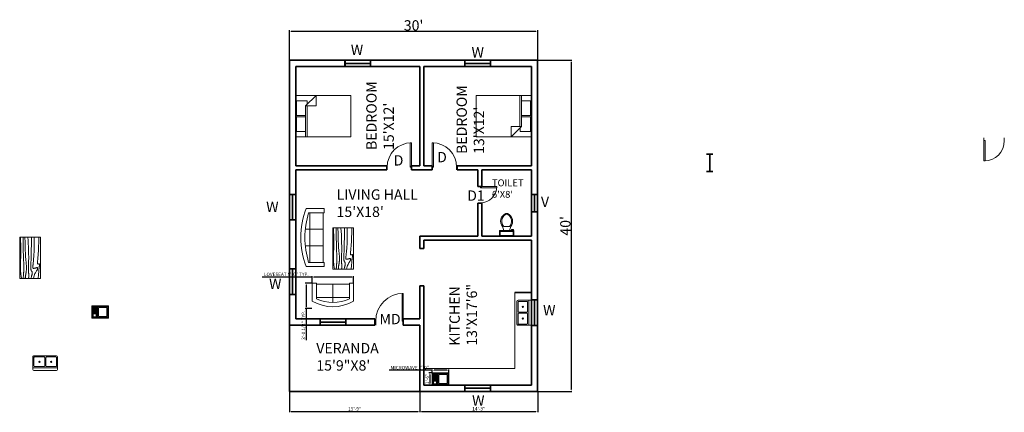
# Model space of a CAD drawing. Units: inches. Extents: x 1662 to 23131, y 1265 to 19127.
# Tile 2 of 26: x 4056 to 5485, y 1980 to 2549. Entities that reach past the tile are written whole.
import ezdxf

# ---------------------------------------------------------------- set-up
doc = ezdxf.new("R2010")
doc.units = ezdxf.units.IN
for name, color, linetype, lineweight in [('A-ANNO-DIMS', 4, 'Continuous', 18), ('A-ANNO-IDEN', 7, 'Continuous', 18), ('A-AREA-IDEN', 7, 'Continuous', 18), ('A-DOOR', 3, 'Continuous', 18), ('A-EQPM', 8, 'Continuous', 18), ('A-FLOR-CASE', 8, 'Continuous', 18), ('A-FLOR-FIXT', 9, 'Continuous', 18), ('A-FURN', 8, 'Continuous', 18), ('A-GLAZ', 4, 'Continuous', 18), ('A-WALL', 7, 'Continuous', 35)]:
    doc.layers.add(name, color=color, linetype=linetype, lineweight=lineweight)
doc.styles.get("Standard").update_dxf_attribs({"font": 'arial.ttf'})
doc.dimstyles.new('ISO-25', dxfattribs={"dimtxt": 5, "dimasz": 2.5, "dimexe": 1.25, "dimexo": 0.625, "dimtad": 1, "dimlunit": 3, "dimtxsty": 'Standard', "dimcen": 2.5, "dimadec": 0, "dimazin": 0, "dimtfac": 1, "dimtmove": 0, "dimatfit": 3, "dimfxl": 1, "dimarcsym": 0})

# ---------------------------------------------------------------- blocks, each defined once
blk = doc.blocks.new('*U25')
for p, q in [((-750, 0), (-750, -100)), ((0, 0), (0, -100))]:
    blk.add_line(p, q)
blk.add_lwpolyline([(0, 0), (0, 750), (-43.75, 750), (-43.75, 0)], close=True)
blk.add_arc((0, 0), 750, 90, 180)
blk = doc.blocks.new('*U26')
for p, q in [((0, 0), (0, -100)), ((900, 0), (900, -100))]:
    blk.add_line(p, q)
blk.add_lwpolyline([(0, 0), (0, 900), (43.75, 900), (43.75, 0)], close=True)
blk.add_arc((0, 0), 900, 0, 90)
blk = doc.blocks.new('*U4')
for p, q in [((0, 0), (0, -100)), ((-900, 0), (-900, -100))]:
    blk.add_line(p, q)
blk.add_lwpolyline([(0, 0), (0, 900), (-43.75, 900), (-43.75, 0)], close=True)
blk.add_arc((0, 0), 900, 90, 180)
blk = doc.blocks.new('*U27')
for p, q in [((0, 0), (0, -6)), ((-40, 0), (-40, -6))]:
    blk.add_line(p, q)
blk.add_lwpolyline([(0, 0), (0, 40), (-1.75, 40), (-1.75, 0)], close=True)
blk.add_arc((0, 0), 40, 90, 180)
blk = doc.blocks.new('*U28')
for p, q in [((0, 0), (0, -100)), ((600, 0), (600, -100))]:
    blk.add_line(p, q)
blk.add_lwpolyline([(0, 0), (0, 600), (43.75, 600), (43.75, 0)], close=True)
blk.add_arc((0, 0), 600, 0, 90)
blk = doc.blocks.new('Toilet - top')
for p, q in [((-10, -8.5), (-8, -8.5)), ((-10, -9.5), (-10, -8.5)), ((-7, -9.5), (-10, -9.5)), ((-8, -8.5), (-8, -8)), ((-7, -8), (-7, -9.5)), ((-4, -8), (-6, -14)), ((4, -14), (-4, -14)), ((4, -8), (6, -14)), ((9.5, -6), (9.5, -2))]:
    blk.add_line(p, q)
blk.add_lwpolyline([(10.5, -8), (10.5, 0), (-10.5, 0), (-10.5, -8)], close=True)
for points in [[(-9.5, -2), (-9.5, -6)], [(8.5, -1), (-8.5, -1)], [(-8.5, -7), (8.5, -7)]]:
    blk.add_lwpolyline(points)
for centre, radius, start, end in [((-8.6, -1.9), 0.884, 81.8699, 188.1301), ((-8.6, -6.1), 0.884, 171.8699, 278.1301), ((3.5, -21.6), 12.2, 141.4691, 247.9714), ((4.2, -21.8), 11.3, 136.3677, 238.9468), ((-3.5, -21.6), 12.2, 292.0284, 38.5307), ((-4.2, -21.8), 11.3, 301.053, 43.6321), ((8.6, -1.9), 0.884, 351.8699, 98.1301), ((8.6, -6.1), 0.884, 261.8699, 8.1301), ((0, -27.9), 4, 245.7318, 294.2682), ((0, -29), 4, 254.8605, 285.1395)]:
    blk.add_arc(centre, radius, start, end)
blk = doc.blocks.new('Bed - Queen')
for p, q in [((0, -80.00003), (0, 0)), ((0, 0), (59.99999, 0)), ((59.99999, 0), (59.99999, -80.00003)), ((7.99999, -1.2), (28.79998, -1.2)), ((7.99999, -14.4), (7.99999, -1.2)), ((28.79998, -1.2), (28.79998, -14.4)), ((31.19999, -1.2), (51.99999, -1.2)), ((31.19999, -14.4), (31.19999, -1.2)), ((51.99999, -1.2), (51.99999, -16.4)), ((0, -14.4), (44.8, -14.4)), ((44.8, -16.8), (0, -16.8)), ((59.99999, -29.6), (44.8, -14.4)), ((44.8, -14.4), (44.8, -29.6)), ((51.99999, -16.4), (46.79936, -16.4)), ((44.8, -29.6), (59.99999, -29.6)), ((59.99999, -80.00003), (0, -80.00003))]:
    blk.add_line(p, q)
blk = doc.blocks.new('Sofa - Roundback 7 ft.')
for p, q in [((-36.000027, -34), (-36.000027, -11.4696)), ((-35.999844, -13.3819), (35.9998, -13.3819)), ((-12.00002, -32.4421), (-12.00003, -6.5971)), ((11.99997, -32.4421), (11.99998, -6.5971)), ((35.99998, -34), (35.99998, -11.4696)), ((-36.000027, -32.4421), (35.99998, -32.4421))]:
    blk.add_line(p, q)
for points in [[(-36.000027, -34), (-42.000027, -34), (-42.000027, -8)], [(41.99998, -8), (41.99998, -34), (35.99998, -34)]]:
    blk.add_lwpolyline(points)
for centre, radius, start, end in [((0, -114.25), 114.25, 68.43141, 111.5686), ((-0.00001, -127.1968), 121.1968, 72.72033, 107.2797)]:
    blk.add_arc(centre, radius, start, end)
blk = doc.blocks.new('Table - Rectangular Woodgrain 60 x 30 in.')
for p, q in [((0, 0), (0, -30)), ((60, 0), (0, 0)), ((60, -30), (60, 0)), ((0, -30), (60, -30))]:
    blk.add_line(p, q)
for points in [[(0, -2.4), (4.8155, -2.418), (9.0302, -2.4688), (12.709, -2.5477), (15.9167, -2.65), (18.7181, -2.7711), (21.1781, -2.9063), (23.3616, -3.0508), (25.3333, -3.2), (27.1477, -3.3495), (28.8172, -3.4958), (30.3437, -3.636), (31.7291, -3.7667), (32.9756, -3.8849), (34.0849, -3.9875), (35.059, -4.0714), (35.9, -4.1334), (36.6114, -4.1711), (37.2041, -4.1854), (37.6906, -4.1779), (38.0833, -4.15), (38.3948, -4.1034), (38.6375, -4.0396), (38.8239, -3.9602), (38.9666, -3.8667), (39.0764, -3.7608), (39.1573, -3.6448), (39.2116, -3.521), (39.2416, -3.3917), (39.2498, -3.2593), (39.2385, -3.1261), (39.21, -2.9944), (39.1666, -2.8667), (39.111, -2.7447), (39.0468, -2.6281), (38.978, -2.5163), (38.9083, -2.4083), (38.8418, -2.3035), (38.7823, -2.201), (38.7337, -2.1001), (38.7, -2), (38.6844, -1.9003), (38.6875, -1.8021), (38.7094, -1.707), (38.75, -1.6167), (38.8094, -1.5326), (38.8875, -1.4563), (38.9844, -1.3893), (39.1, -1.3333), (39.2351, -1.2896), (39.3937, -1.2583), (39.5804, -1.2396), (39.8, -1.2333), (40.057, -1.2396), (40.3562, -1.2583), (40.7023, -1.2896), (41.1, -1.3333), (41.5547, -1.3895), (42.0755, -1.4573), (42.6721, -1.5361), (43.3542, -1.625), (44.1316, -1.7233), (45.014, -1.8302), (46.0114, -1.9449), (47.1333, -2.0667), (48.3862, -2.1947), (49.7625, -2.3281), (51.2513, -2.4663), (52.8416, -2.6083), (54.5226, -2.7535), (56.2833, -2.9011), (58.1127, -3.0501), (60, -3.2)], [(0, -9.2), (6.5759, -9.0858), (11.9385, -9.0365), (16.2527, -9.0418), (19.6833, -9.0917), (22.3952, -9.1759), (24.5531, -9.2844), (26.322, -9.4069), (27.8666, -9.5333), (29.3241, -9.6553), (30.7203, -9.7719), (32.0532, -9.8837), (33.3208, -9.9917), (34.5213, -10.0965), (35.6526, -10.199), (36.7128, -10.2999), (37.7, -10.4), (38.6129, -10.4996), (39.4531, -10.5969), (40.223, -10.6895), (40.925, -10.775), (41.5613, -10.8512), (42.1344, -10.9156), (42.6465, -10.966), (43.1, -11), (43.4976, -11.0158), (43.8437, -11.0136), (44.143, -10.9942), (44.4, -10.9583), (44.6195, -10.9069), (44.8062, -10.8406), (44.9648, -10.7603), (45.1, -10.6667), (45.2155, -10.5598), (45.3114, -10.4365), (45.3871, -10.2929), (45.4416, -10.125), (45.4743, -9.929), (45.4844, -9.7011), (45.4709, -9.4371), (45.4333, -9.1333), (45.3716, -8.7883), (45.2896, -8.4104), (45.1919, -8.0107), (45.0833, -7.6), (44.9685, -7.1893), (44.8521, -6.7896), (44.7388, -6.4117), (44.6333, -6.0667), (44.54, -5.7628), (44.4614, -5.4979), (44.4001, -5.2675), (44.3583, -5.0667), (44.3384, -4.8909), (44.3427, -4.7354), (44.3736, -4.5956), (44.4333, -4.4667), (44.5236, -4.3453), (44.6427, -4.2333), (44.7884, -4.1339), (44.9583, -4.05), (45.1501, -3.9849), (45.3614, -3.9417), (45.59, -3.9234), (45.8333, -3.9333), (46.0915, -3.9749), (46.3734, -4.0531), (46.6906, -4.1736), (47.0542, -4.3417), (47.4756, -4.5629), (47.9661, -4.8427), (48.5372, -5.1866), (49.2, -5.6), (49.9676, -6.0844), (50.8594, -6.625), (51.8965, -7.2031), (53.1, -7.8), (54.491, -8.3969), (56.0906, -8.975), (57.9199, -9.5156), (60, -10)], [(0, -12.8), (5.1847, -12.9322), (9.6213, -13.0323), (13.3963, -13.1059), (16.5958, -13.1583), (19.3063, -13.1952), (21.614, -13.2219), (23.6054, -13.2439), (25.3666, -13.2667), (26.9728, -13.2947), (28.4531, -13.3281), (29.8256, -13.3663), (31.1083, -13.4083), (32.3191, -13.4535), (33.476, -13.501), (34.597, -13.5501), (35.7, -13.6), (36.7984, -13.6497), (37.8875, -13.6979), (38.9578, -13.743), (40, -13.7833), (41.0047, -13.8174), (41.9625, -13.8438), (42.864, -13.8607), (43.7, -13.8667), (44.4631, -13.8604), (45.1552, -13.8417), (45.7801, -13.8104), (46.3416, -13.7667), (46.8439, -13.7104), (47.2906, -13.6417), (47.6858, -13.5604), (48.0333, -13.4667), (48.3375, -13.3608), (48.6042, -13.2448), (48.8396, -13.121), (49.05, -12.9917), (49.2417, -12.8593), (49.4208, -12.7261), (49.5937, -12.5944), (49.7667, -12.4667), (49.9452, -12.3451), (50.1323, -12.2313), (50.3303, -12.1268), (50.5416, -12.0333), (50.7686, -11.9524), (51.0135, -11.8854), (51.2788, -11.8341), (51.5666, -11.8), (51.8785, -11.7843), (52.2116, -11.7865), (52.562, -11.8059), (52.926, -11.8417), (53.2998, -11.8931), (53.6795, -11.9594), (54.0614, -12.0397), (54.4416, -12.1333), (54.8223, -12.2401), (55.2293, -12.3625), (55.6942, -12.5037), (56.2489, -12.6667), (56.9251, -12.8547), (57.7545, -13.0708), (58.7689, -13.3182), (60, -13.6)], [(0, -18), (5.124, -17.7273), (9.6609, -17.5057), (13.6705, -17.3303), (17.2125, -17.1958), (20.3467, -17.0973), (23.1328, -17.0297), (25.6307, -16.9878), (27.9, -16.9667), (29.9928, -16.9617), (31.9302, -16.9703), (33.7254, -16.9907), (35.3917, -17.0208), (36.9423, -17.0588), (38.3906, -17.1026), (39.7499, -17.1503), (41.0333, -17.2), (42.2519, -17.2496), (43.4073, -17.2969), (44.4986, -17.3395), (45.525, -17.375), (46.4858, -17.4012), (47.3802, -17.4156), (48.2074, -17.416), (48.9667, -17.4), (49.6583, -17.3662), (50.2872, -17.3167), (50.8595, -17.2547), (51.3812, -17.1833), (51.8584, -17.1057), (52.2971, -17.025), (52.7034, -16.9443), (53.0833, -16.8667), (53.443, -16.7951), (53.789, -16.7313), (54.128, -16.6768), (54.4666, -16.6334), (54.8115, -16.6024), (55.1693, -16.5854), (55.5465, -16.5841), (55.95, -16.6), (56.3828, -16.6337), (56.8346, -16.6823), (57.2915, -16.7418), (57.7396, -16.8084), (58.165, -16.878), (58.5539, -16.9469), (58.8924, -17.0111), (59.1666, -17.0667), (59.3679, -17.1107), (59.5078, -17.1438), (59.6032, -17.1675), (59.6708, -17.1833), (59.7275, -17.193), (59.7901, -17.1979), (59.8753, -17.1998), (60, -17.2)], [(0, -22.4), (8.0098, -22.2501), (14.4094, -22.1011), (19.4168, -21.9535), (23.25, -21.8083), (26.1269, -21.6663), (28.2656, -21.5281), (29.884, -21.3947), (31.2, -21.2667), (32.3967, -21.1448), (33.5172, -21.0292), (34.5697, -20.9198), (35.5625, -20.8167), (36.5037, -20.7198), (37.4015, -20.6292), (38.2642, -20.5448), (39.1, -20.4667), (39.9164, -20.3951), (40.7187, -20.3313), (41.5117, -20.2768), (42.3, -20.2333), (43.0883, -20.2024), (43.8812, -20.1854), (44.6836, -20.1841), (45.5, -20.2), (46.3328, -20.234), (47.1747, -20.2844), (48.0163, -20.3488), (48.8479, -20.425), (49.66, -20.5106), (50.4429, -20.6031), (51.1872, -20.7004), (51.8833, -20.8), (52.5246, -20.8999), (53.1166, -20.9995), (53.6681, -21.0983), (54.1875, -21.1958), (54.6834, -21.2919), (55.1646, -21.3859), (55.6394, -21.4777), (56.1167, -21.5667), (56.6028, -21.6515), (57.0961, -21.7266), (57.5929, -21.7852), (58.0896, -21.8208), (58.5823, -21.8268), (59.0674, -21.7964), (59.5412, -21.723), (60, -21.6)], [(0, -25.2), (8.6355, -25.0504), (15.7026, -24.9031), (21.4049, -24.7606), (25.9458, -24.625), (29.529, -24.4988), (32.3578, -24.3844), (34.6359, -24.284), (36.5667, -24.2), (38.3213, -24.1341), (39.9417, -24.0854), (41.437, -24.0523), (42.8167, -24.0333), (44.0901, -24.0268), (45.2667, -24.0313), (46.3557, -24.0451), (47.3667, -24.0667), (48.309, -24.0947), (49.1928, -24.1287), (50.0284, -24.168), (50.826, -24.2125), (51.5959, -24.2617), (52.3483, -24.3151), (53.0935, -24.3725), (53.8417, -24.4334), (54.6009, -24.497), (55.3699, -24.561), (56.1454, -24.6226), (56.9239, -24.6792), (57.7021, -24.7279), (58.4764, -24.7662), (59.2435, -24.7911), (60, -24.8)], [(0, -28.8), (5.6867, -28.6681), (10.45, -28.5698), (14.407, -28.5012), (17.675, -28.4584), (20.3711, -28.4374), (22.6125, -28.4344), (24.5164, -28.4455), (26.2, -28.4667), (27.762, -28.4947), (29.2276, -28.5281), (30.6033, -28.5663), (31.8958, -28.6084), (33.1118, -28.6535), (34.2578, -28.7011), (35.3405, -28.7501), (36.3666, -28.8), (37.3443, -28.8497), (38.288, -28.8974), (39.2137, -28.9412), (40.1375, -28.9792), (41.0753, -29.0093), (42.0432, -29.0297), (43.0572, -29.0384), (44.1333, -29.0333), (45.2936, -29.0114), (46.5843, -28.9641), (48.0579, -28.8816), (49.7666, -28.7542), (51.7629, -28.5721), (54.0989, -28.3255), (56.8272, -28.0048), (60, -27.6)]]:
    blk.add_lwpolyline(points)
blk = doc.blocks.new('Sofa - Roundback Loveseat 5 ft.')
for p, q in [((-24, -33.99998), (-24, -11.46958)), ((-23.9998, -13.38178), (23.99986, -13.38178)), ((0, -32.44198), (0, -5.99998)), ((24.00004, -33.99998), (24.00004, -11.46958)), ((-24, -32.44198), (24.00004, -32.44198))]:
    blk.add_line(p, q)
for points in [[(-24, -33.99998), (-30, -33.99998), (-30, -7.99998)], [(30.00004, -7.99998), (30.00004, -33.99998), (24.00004, -33.99998)]]:
    blk.add_lwpolyline(points)
for centre, radius, start, end in [((0, -60.24998), 60.24998, 60.13715, 119.8628), ((0, -61.38438), 55.38444, 64.32083, 115.6792)]:
    blk.add_arc(centre, radius, start, end)
blk = doc.blocks.new('Sink-double - 36 in top')
for p, q in [((-18, -4), (18, -4)), ((-0.75, -18.5), (-0.75, -6.5)), ((0.75, -6.5), (0.75, -18.5))]:
    blk.add_line(p, q)
for points in [[(-16.5, 0), (16.5, 0)], [(-18, -19.5), (-18, -1.5)], [(-16.5, -18.5), (-16.5, -6.5)], [(-15.5, -5.5), (-1.75, -5.5)], [(1.75, -5.5), (15.5, -5.5)], [(16.5, -6.5), (16.5, -18.5)], [(18, -1.5), (18, -19.5)], [(16.5, -21), (-16.5, -21)], [(-1.75, -19.5), (-15.5, -19.5)], [(15.5, -19.5), (1.75, -19.5)]]:
    blk.add_lwpolyline(points)
for centre, radius in [((-8.5, -12.5), 1), ((-8.5, -12.5), 0.5), ((8.5, -12.5), 1), ((8.5, -12.5), 0.5)]:
    blk.add_circle(centre, radius)
for centre, radius, start, end in [((-16.5, -1.5), 1.5, 90, 180), ((16.5, -1.5), 1.5, 0, 90), ((-15.5, -6.5), 1, 90, 180), ((-1.75, -6.5), 1, 0, 90), ((1.75, -6.5), 1, 90, 180), ((15.5, -6.5), 1, 0, 90), ((-16.5, -19.5), 1.5, 180, 270), ((-15.5, -18.5), 1, 180, 270), ((-1.75, -18.5), 1, 270, 0), ((1.75, -18.5), 1, 180, 270), ((15.5, -18.5), 1, 270, 0), ((16.5, -19.5), 1.5, 270, 0)]:
    blk.add_arc(centre, radius, start, end)
blk = doc.blocks.new('Microwave')
for p, q in [((18, 10), (22, 10)), ((22, 9), (18, 9)), ((18, 8), (22, 8)), ((22, 7), (18, 7)), ((20, 6), (18, 6)), ((19, 7), (19, 11)), ((19, 6), (19, 7)), ((20, 11), (20, 7)), ((20, 7), (20, 6)), ((21, 7), (21, 11))]:
    blk.add_line(p, q)
for points in [[(0, 0), (0, 18), (24, 18), (24, 0)], [(1, 1), (1, 17), (16, 17), (16, 1)], [(2.5, 2.5), (2.5, 15.5), (14.5, 15.5), (14.5, 2.5)], [(17, 1), (17, 17), (23, 17), (23, 1)], [(18, 12), (18, 16), (22, 16), (22, 12)], [(18, 2), (18, 11), (22, 11), (22, 2)], [(18.5, 4.5), (18.5, 5.5), (21.5, 5.5), (21.5, 4.5)], [(18.5, 3), (18.5, 4), (21.5, 4), (21.5, 3)]]:
    blk.add_lwpolyline(points, close=True)
blk = doc.blocks.new('*D31')
at = {"layer": 'A-ANNO-DIMS', "color": 0, "lineweight": -2, "transparency": 16777216}
for p, q in [((4447.9, 2490.6), (4447.9, 2533.6)), ((4450.4, 2532.3), (4805.4, 2532.3)), ((4807.9, 2490.6), (4807.9, 2533.6))]:
    blk.add_line(p, q, dxfattribs=at)
at = {"layer": 'A-ANNO-DIMS', "color": 0, "transparency": 16777216}
for points in [[(4450.4, 2532.7), (4450.4, 2531.9), (4447.9, 2532.3)], [(4805.4, 2532.7), (4805.4, 2531.9), (4807.9, 2532.3)]]:
    blk.add_solid(points, dxfattribs=at)
at = {"layer": 'Defpoints', "color": 0, "transparency": 16777216}
for p in [(4807.9, 2532.3), (4447.9, 2490), (4807.9, 2490)]:
    blk.add_point(p, dxfattribs=at)
at = {"layer": 'A-ANNO-DIMS', "color": 0, "transparency": 16777216, "insert": (4627.9, 2540.6), "char_height": 5, "attachment_point": 5}
blk.add_mtext("{\\H3x;30'}", dxfattribs=at)
blk = doc.blocks.new('*D32')
at = {"layer": 'A-ANNO-DIMS', "color": 0, "lineweight": -2, "transparency": 16777216}
for p, q in [((4808.5, 2490), (4857.6, 2490)), ((4856.3, 2487.5), (4856.3, 2012.5)), ((4808.5, 2010), (4857.6, 2010))]:
    blk.add_line(p, q, dxfattribs=at)
at = {"layer": 'A-ANNO-DIMS', "color": 0, "transparency": 16777216}
for points in [[(4855.9, 2487.5), (4856.8, 2487.5), (4856.3, 2490)], [(4855.9, 2012.5), (4856.8, 2012.5), (4856.3, 2010)]]:
    blk.add_solid(points, dxfattribs=at)
at = {"layer": 'Defpoints', "color": 0, "transparency": 16777216}
for p in [(4807.9, 2490), (4807.9, 2010), (4856.3, 2010)]:
    blk.add_point(p, dxfattribs=at)
at = {"layer": 'A-ANNO-DIMS', "color": 0, "transparency": 16777216, "insert": (4848.1, 2250), "char_height": 5, "attachment_point": 5, "rotation": 90}
blk.add_mtext("{\\H3x;40'}", dxfattribs=at)
blk = doc.blocks.new('WIN-36-J9X1')
for p, q in [((0, 9), (0, 0)), ((1, 9), (1, 0)), ((1, 5), (37, 5)), ((1, 4.5), (37, 4.5)), ((1, 4), (37, 4)), ((37, 9), (37, 0)), ((38, 9), (38, 0))]:
    blk.add_line(p, q)
blk = doc.blocks.new('VENT-24-J9X1')
for p, q in [((0, 9), (0, 0)), ((1, 9), (1, 0)), ((1, 5), (25, 5)), ((1, 4.5), (25, 4.5)), ((1, 4), (25, 4)), ((25, 9), (25, 0)), ((26, 9), (26, 0))]:
    blk.add_line(p, q)
blk = doc.blocks.new('*D185')
at = {"layer": 'A-ANNO-DIMS', "color": 0, "lineweight": -2, "transparency": 16777216}
for p, q in [((4480.9, 2175.8), (4408.1, 2175.8)), ((4480.9, 2167.4), (4480.9, 2177)), ((4538.4, 2175.8), (4483.4, 2175.8)), ((4540.9, 2167.4), (4540.9, 2177))]:
    blk.add_line(p, q, dxfattribs=at)
at = {"layer": 'A-ANNO-DIMS', "color": 0, "transparency": 16777216}
for points in [[(4483.4, 2176.2), (4483.4, 2175.3), (4480.9, 2175.8)], [(4538.4, 2176.2), (4538.4, 2175.3), (4540.9, 2175.8)]]:
    blk.add_solid(points, dxfattribs=at)
at = {"layer": 'Defpoints', "color": 0, "transparency": 16777216}
for p in [(4480.9, 2175.8), (4480.9, 2166.8), (4540.9, 2166.8)]:
    blk.add_point(p, dxfattribs=at)
at = {"layer": 'A-ANNO-DIMS', "color": 0, "transparency": 16777216, "insert": (4443.2, 2179), "char_height": 5, "attachment_point": 5}
blk.add_mtext('LOVESEAT 5\'-0" TYP.', dxfattribs=at)
blk = doc.blocks.new('*D186')
at = {"layer": 'A-ANNO-DIMS', "color": 0, "lineweight": -2, "transparency": 16777216}
for p, q in [((4480.3, 2166.8), (4470.6, 2166.8)), ((4471.9, 2164.3), (4471.9, 2132.6)), ((4480.3, 2130.1), (4470.6, 2130.1)), ((4471.9, 2130.1), (4471.9, 2084.2))]:
    blk.add_line(p, q, dxfattribs=at)
at = {"layer": 'A-ANNO-DIMS', "color": 0, "transparency": 16777216}
for points in [[(4471.5, 2164.3), (4472.3, 2164.3), (4471.9, 2166.8)], [(4471.5, 2132.6), (4472.3, 2132.6), (4471.9, 2130.1)]]:
    blk.add_solid(points, dxfattribs=at)
at = {"layer": 'Defpoints', "color": 0, "transparency": 16777216}
for p in [(4480.9, 2166.8), (4471.9, 2130.1), (4480.9, 2130.1)]:
    blk.add_point(p, dxfattribs=at)
at = {"layer": 'A-ANNO-DIMS', "color": 0, "transparency": 16777216, "insert": (4468.7, 2105.9), "char_height": 5, "attachment_point": 5, "rotation": 90}
blk.add_mtext('3\'-0 1/2" TYP.', dxfattribs=at)
blk = doc.blocks.new('*D189')
at = {"layer": 'A-ANNO-DIMS', "color": 0, "lineweight": -2, "transparency": 16777216}
for p, q in [((4655, 2040.6), (4592.4, 2040.6)), ((4655, 2037.6), (4655, 2041.9)), ((4676.5, 2040.6), (4657.5, 2040.6)), ((4679, 2037.6), (4679, 2041.9))]:
    blk.add_line(p, q, dxfattribs=at)
at = {"layer": 'A-ANNO-DIMS', "color": 0, "transparency": 16777216}
for points in [[(4657.5, 2041), (4657.5, 2040.2), (4655, 2040.6)], [(4676.5, 2041), (4676.5, 2040.2), (4679, 2040.6)]]:
    blk.add_solid(points, dxfattribs=at)
at = {"layer": 'Defpoints', "color": 0, "transparency": 16777216}
for p in [(4655, 2040.6), (4655, 2037), (4679, 2037)]:
    blk.add_point(p, dxfattribs=at)
at = {"layer": 'A-ANNO-DIMS', "color": 0, "transparency": 16777216, "insert": (4622.4, 2043.8), "char_height": 5, "attachment_point": 5}
blk.add_mtext('MICROWAVE 2\'-0"', dxfattribs=at)
blk = doc.blocks.new('*D190')
at = {"layer": 'A-ANNO-DIMS', "color": 0, "lineweight": -2, "transparency": 16777216}
for p, q in [((4654.3, 2037), (4650.1, 2037)), ((4651.4, 2034.5), (4651.4, 2021.5)), ((4654.3, 2019), (4650.1, 2019))]:
    blk.add_line(p, q, dxfattribs=at)
at = {"layer": 'A-ANNO-DIMS', "color": 0, "transparency": 16777216}
for points in [[(4650.9, 2034.5), (4651.8, 2034.5), (4651.4, 2037)], [(4650.9, 2021.5), (4651.8, 2021.5), (4651.4, 2019)]]:
    blk.add_solid(points, dxfattribs=at)
at = {"layer": 'Defpoints', "color": 0, "transparency": 16777216}
for p in [(4655, 2037), (4651.4, 2019), (4655, 2019)]:
    blk.add_point(p, dxfattribs=at)
at = {"layer": 'A-ANNO-DIMS', "color": 0, "transparency": 16777216, "insert": (4648.2, 2028), "char_height": 5, "attachment_point": 5, "rotation": 90}
blk.add_mtext('1\'-6"', dxfattribs=at)
blk = doc.blocks.new('*D205')
at = {"layer": 'A-ANNO-DIMS', "color": 0, "lineweight": -2, "transparency": 16777216}
for p, q in [((4447.9, 2009.4), (4447.9, 1979.7)), ((4636.9, 2009.4), (4636.9, 1979.7)), ((4450.4, 1980.9), (4634.4, 1980.9))]:
    blk.add_line(p, q, dxfattribs=at)
at = {"layer": 'A-ANNO-DIMS', "color": 0, "transparency": 16777216}
for points in [[(4450.4, 1981.3), (4450.4, 1980.5), (4447.9, 1980.9)], [(4634.4, 1981.3), (4634.4, 1980.5), (4636.9, 1980.9)]]:
    blk.add_solid(points, dxfattribs=at)
at = {"layer": 'Defpoints', "color": 0, "transparency": 16777216}
for p in [(4447.9, 2010), (4636.9, 2010), (4636.9, 1980.9)]:
    blk.add_point(p, dxfattribs=at)
at = {"layer": 'A-ANNO-DIMS', "color": 0, "transparency": 16777216, "insert": (4542.4, 1984.1), "char_height": 5, "attachment_point": 5}
blk.add_mtext('15\'-9"', dxfattribs=at)
blk = doc.blocks.new('*D206')
at = {"layer": 'A-ANNO-DIMS', "color": 0, "lineweight": -2, "transparency": 16777216}
for p, q in [((4636.9, 2009.4), (4636.9, 1979.7)), ((4807.9, 2009.4), (4807.9, 1979.7)), ((4639.4, 1980.9), (4805.4, 1980.9))]:
    blk.add_line(p, q, dxfattribs=at)
at = {"layer": 'A-ANNO-DIMS', "color": 0, "transparency": 16777216}
for points in [[(4639.4, 1981.3), (4639.4, 1980.5), (4636.9, 1980.9)], [(4805.4, 1981.3), (4805.4, 1980.5), (4807.9, 1980.9)]]:
    blk.add_solid(points, dxfattribs=at)
at = {"layer": 'Defpoints', "color": 0, "transparency": 16777216}
for p in [(4636.9, 2010), (4807.9, 2010), (4807.9, 1980.9)]:
    blk.add_point(p, dxfattribs=at)
at = {"layer": 'A-ANNO-DIMS', "color": 0, "transparency": 16777216, "insert": (4722.4, 1984.1), "char_height": 5, "attachment_point": 5}
blk.add_mtext('14\'-3"', dxfattribs=at)

msp = doc.modelspace()

# ---------------------------------------------------------------- linework, layer by layer
at = {"layer": 'A-FLOR-CASE'}
for p, q in [((4774.881, 2153.333), (4774.881, 2043.019)), ((4774.881, 2043.019), (4642.881, 2043.019))]:
    msp.add_line(p, q, dxfattribs=at)
at = {"layer": 'A-WALL'}
for p, q in [((4447.881, 2490.019), (4807.881, 2490.019)), ((4447.881, 2106.019), (4447.881, 2490.019)), ((4807.881, 2490.019), (4807.881, 2010.019)), ((4456.881, 2481.019), (4636.881, 2481.019)), ((4456.881, 2337.019), (4456.881, 2481.019)), ((4636.881, 2337.019), (4636.881, 2481.019)), ((4642.881, 2337.019), (4642.881, 2481.019)), ((4642.881, 2481.019), (4798.881, 2481.019)), ((4798.881, 2481.019), (4798.881, 2337.019)), ((4456.881, 2337.019), (4588.881, 2337.019)), ((4456.881, 2115.019), (4456.881, 2331.019)), ((4456.881, 2331.019), (4588.881, 2331.019)), ((4588.881, 2337.019), (4588.881, 2331.019)), ((4624.881, 2337.019), (4624.881, 2331.019)), ((4624.881, 2337.019), (4636.881, 2337.019)), ((4624.881, 2331.019), (4654.881, 2331.019)), ((4642.881, 2337.019), (4654.881, 2337.019)), ((4654.881, 2331.019), (4654.881, 2337.019)), ((4690.881, 2331.019), (4690.881, 2337.019)), ((4690.881, 2337.019), (4798.881, 2337.019)), ((4690.881, 2331.019), (4720.881, 2331.019)), ((4720.881, 2331.019), (4720.881, 2307.019)), ((4726.881, 2331.019), (4726.881, 2307.019)), ((4726.881, 2331.019), (4798.881, 2331.019)), ((4798.881, 2331.019), (4798.881, 2235.019)), ((4798.881, 2331.019), (4798.881, 2235.019)), ((4720.881, 2307.019), (4726.881, 2307.019)), ((4720.881, 2283.019), (4726.881, 2283.019)), ((4720.881, 2283.019), (4720.881, 2235.019)), ((4726.881, 2283.019), (4726.881, 2235.019)), ((4636.881, 2235.019), (4720.881, 2235.019)), ((4636.881, 2217.019), (4636.881, 2235.019)), ((4642.881, 2229.019), (4798.881, 2229.019)), ((4642.881, 2217.019), (4642.881, 2229.019)), ((4726.881, 2235.019), (4798.881, 2235.019)), ((4798.881, 2229.019), (4798.881, 2019.019)), ((4798.881, 2229.019), (4798.881, 2019.019)), ((4636.881, 2217.019), (4642.881, 2217.019)), ((4636.881, 2115.019), (4636.881, 2163.019)), ((4636.881, 2163.019), (4642.881, 2163.019)), ((4642.881, 2019.019), (4642.881, 2163.019)), ((4798.881, 2153.333), (4774.881, 2153.333)), ((4456.881, 2115.019), (4571.799, 2115.019)), ((4510.881, 2115.019), (4510.881, 2115.019)), ((4510.881, 2115.019), (4510.881, 2115.019)), ((4571.799, 2106.019), (4571.799, 2115.019)), ((4612.881, 2115.019), (4636.881, 2115.019)), ((4612.881, 2106.019), (4612.881, 2115.019)), ((4612.881, 2115.019), (4636.881, 2115.019)), ((4447.881, 2106.019), (4571.799, 2106.019)), ((4447.881, 2106.019), (4447.881, 2010.019)), ((4612.881, 2106.019), (4636.881, 2106.019)), ((4636.881, 2010.019), (4636.881, 2106.019)), ((4798.881, 2019.019), (4642.881, 2019.019)), ((4807.881, 2010.019), (4447.881, 2010.019))]:
    msp.add_line(p, q, dxfattribs=at)

# ---------------------------------------------------------------- block references
at = {"layer": 'A-DOOR', "xscale": 0.0393700787401575, "yscale": 0.0393700787401575, "zscale": 0.0393700787401575}
for name, p, rotation in [('*U25', (5455.342, 2373.57), 180), ('*U28', (4724.818, 2307.019), 270)]:
    msp.add_blockref(name, p, dxfattribs=dict(at, rotation=rotation))
for name, p in [('*U4', (4624.881, 2334.956)), ('*U26', (4654.881, 2334.956))]:
    msp.add_blockref(name, p, dxfattribs=at)
at = {"layer": 'A-DOOR'}
msp.add_blockref('*U27', (4612.881, 2112.019), dxfattribs=at)
at = {"layer": 'A-EQPM', "rotation": 180}
for p in [(4185.257, 2134.188), (4678.961, 2037.019)]:
    msp.add_blockref('Microwave', p, dxfattribs=at)
at = {"layer": 'A-FLOR-FIXT'}
for name, p, rotation in [('Toilet - top', (4762.881, 2235.019), 180), ('Sink-double - 36 in top', (4798.881, 2124.019), 270), ('Sink-double - 36 in top', (4093.467, 2040.345), 180)]:
    msp.add_blockref(name, p, dxfattribs=dict(at, rotation=rotation))
at = {"layer": 'A-FURN'}
for name, p, rotation in [('Bed - Queen', (4456.881, 2379.019), 89.99999999999999), ('Bed - Queen', (4798.881, 2439.019), 270), ('Sofa - Roundback 7 ft.', (4464.179, 2233.065), 89.99999999999996), ('Table - Rectangular Woodgrain 60 x 30 in.', (4540.571, 2247.028), 270), ('Table - Rectangular Woodgrain 60 x 30 in.', (4086.438, 2233.807), 270), ('Sofa - Roundback Loveseat 5 ft.', (4510.881, 2132.764), 180)]:
    msp.add_blockref(name, p, dxfattribs=dict(at, rotation=rotation))
at = {"layer": 'A-GLAZ'}
for p in [(4527.881, 2481.019), (4701.881, 2481.019), (4491.881, 2106.019), (4701.881, 2010.019)]:
    msp.add_blockref('WIN-36-J9X1', p, dxfattribs=at)
at = {"layer": 'A-GLAZ', "rotation": 90}
for name, p in [('VENT-24-J9X1', (5061.988, 2328.409)), ('WIN-36-J9X1', (4456.881, 2258.019)), ('VENT-24-J9X1', (4807.881, 2270.019)), ('WIN-36-J9X1', (4456.881, 2150.019)), ('WIN-36-J9X1', (4807.881, 2105.019))]:
    msp.add_blockref(name, p, dxfattribs=at)

# ---------------------------------------------------------------- texts
at = {"layer": 'A-ANNO-IDEN', "char_height": 15, "attachment_point": 1}
for s, heights, insert in [('W', [20], (4536.806, 2512.75)), ('W', [20], (4711.982, 2509.062)), ('D', [0], (4662.013, 2357.104)), ('D', [0], (4599.026, 2352.409)), ('D1', [20], (4705.658, 2301.367)), ('V', [20], (4812.646, 2292.35)), ('W', [20], (4414.038, 2285.015)), ('W', [20], (4418.239, 2173.507)), ('W', [20], (4815.767, 2135.152)), ('MD', [0], (4578.411, 2122.325)), ('W', [20], (4712.798, 2004.096))]:
    msp.add_mtext_dynamic_manual_height_columns(s, width=1142.59551, gutter_width=12.5, heights=heights, dxfattribs=dict(at, insert=insert))
at = {"layer": 'A-AREA-IDEN', "char_height": 15, "attachment_point": 1, "rotation": 90}
for s, insert in [("BEDROOM\\P15'X12'", (4559.243, 2360.011)), ("BEDROOM\\P13'X12'", (4690.206, 2354.293)), ('KITCHEN\\P13\'X17\'6"', (4679.879, 2076.222))]:
    msp.add_mtext_dynamic_manual_height_columns(s, width=1142.59551, gutter_width=12.5, heights=[277.772], dxfattribs=dict(at, insert=insert))
at = {"layer": 'A-AREA-IDEN', "attachment_point": 1}
for s, insert, char_height in [("TOILET\\P6'X8'", (4741.521, 2317.371), 10), ("LIVING HALL\\P15'X18'", (4516.169, 2302.878), 15), ('VERANDA\\P15\'9"X8\'', (4486.77, 2080.107), 15)]:
    msp.add_mtext_dynamic_manual_height_columns(s, width=1142.59551, gutter_width=12.5, heights=[277.772], dxfattribs=dict(at, insert=insert, char_height=char_height))

# ---------------------------------------------------------------- dimensions: what is measured, and where the dimension line sits
at = {"layer": 'A-ANNO-DIMS'}
dim = msp.add_linear_dim(base=(4807.881, 2532.31), p1=(4447.881, 2490.019), p2=(4807.881, 2490.019), text='{\\H3x;<>}', dimstyle='ISO-25', override={"dimclrd": 0, "dimclre": 0, "dimclrt": 0}, dxfattribs=at)
dim.commit()
dim.dimension.update_dxf_attribs({"geometry": '*D31', "text_midpoint": (4627.881, 2540.599)})
for base, p1, p2, angle, text, override, picture, middle in [((4856.348, 2010.019), (4807.881, 2490.019), (4807.881, 2010.019), 90, '{\\H3x;<>}', {"dimclrd": 0, "dimclre": 0, "dimclrt": 0}, '*D32', (4848.065, 2250.019)), ((4480.881, 2175.764), (4540.881, 2166.764), (4480.881, 2166.764), 180, 'LOVESEAT <> TYP.', {"dimdec": 1, "dimlfac": 1, "dimrnd": 0, "dimzin": 1, "dimdsep": 46, "dimlunit": 4, "dimfrac": 2}, '*D185', (4443.218, 2178.976)), ((4471.881, 2130.097), (4480.881, 2166.764), (4480.881, 2130.097), 270, '<> TYP.', {"dimdec": 1, "dimlfac": 1, "dimrnd": 0, "dimzin": 1, "dimdsep": 46, "dimlunit": 4, "dimfrac": 2}, '*D186', (4468.669, 2105.91)), ((4654.961, 2040.619), (4678.961, 2037.019), (4654.961, 2037.019), 180, 'MICROWAVE <>', {"dimdec": 1, "dimlfac": 1, "dimrnd": 0, "dimzin": 1, "dimdsep": 46, "dimlunit": 4, "dimfrac": 2}, '*D189', (4622.409, 2043.831))]:
    dim = msp.add_linear_dim(base=base, p1=p1, p2=p2, angle=angle, text=text, dimstyle='ISO-25', override=override, dxfattribs=at)
    dim.commit()
    dim.dimension.update_dxf_attribs({"geometry": picture, "text_midpoint": middle})
dim = msp.add_linear_dim(base=(4651.361, 2019.019), p1=(4654.961, 2037.019), p2=(4654.961, 2019.019), angle=270, dimstyle='ISO-25', override={"dimdec": 1, "dimlfac": 1, "dimrnd": 0, "dimzin": 1, "dimdsep": 46, "dimlunit": 4, "dimfrac": 2}, dxfattribs=at)
dim.commit()
dim.dimension.update_dxf_attribs({"geometry": '*D190', "text_midpoint": (4648.183, 2028.019)})
for base, p1, p2, picture, middle in [((4636.881, 1980.919), (4447.881, 2010.019), (4636.881, 2010.019), '*D205', (4542.381, 1984.097)), ((4807.881, 1980.919), (4636.881, 2010.019), (4807.881, 2010.019), '*D206', (4722.381, 1984.099))]:
    dim = msp.add_linear_dim(base=base, p1=p1, p2=p2, dimstyle='ISO-25', override={"dimdec": 1, "dimlfac": 1, "dimrnd": 0, "dimzin": 1, "dimdsep": 46, "dimlunit": 4, "dimfrac": 2}, dxfattribs=at)
    dim.commit()
    dim.dimension.update_dxf_attribs({"geometry": picture, "text_midpoint": middle})

doc.saveas('drawing.dxf')
